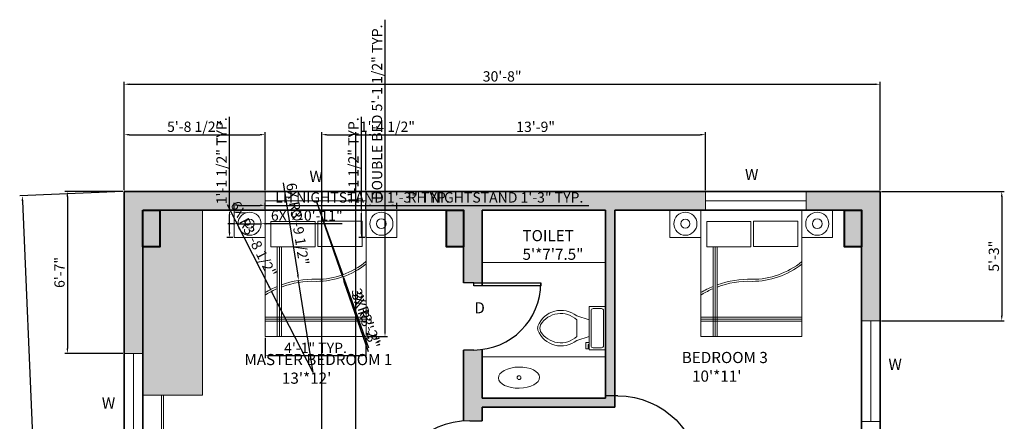
# Model space of a CAD drawing. Units: inches. Extents: x 351 to 1945, y 4338 to 4989.
# Tile 3 of 4: x 351 to 830, y 4716 to 4912. Entities that reach past the tile are written whole.
import ezdxf

# ---------------------------------------------------------------- set-up
doc = ezdxf.new("R2010")
doc.units = ezdxf.units.IN
for name, color, linetype, lineweight in [('A-ANNO-DIMS', 55, 'Continuous', 18), ('A-ANNO-IDEN', 55, 'Continuous', 18), ('A-AREA-IDEN', 55, 'Continuous', 18), ('A-COLS-PATT', 210, 'Continuous', 13), ('A-FLOR-CASE', 30, 'Continuous', 20), ('A-FLOR-CASE-PATT', 30, 'Continuous', 13), ('A-FLOR-FIXT', 9, 'Continuous', 18), ('A-WALL-PATT', 130, 'Continuous', 13), ('COLUMN', 210, 'Continuous', 40), ('DOOR', 52, 'Continuous', 25), ('FUR', 142, 'Continuous', 18), ('WALL', 130, 'Continuous', 35), ('WIND', 10, 'Continuous', 20)]:
    doc.layers.add(name, color=color, linetype=linetype, lineweight=lineweight)
doc.styles.get("Standard").update_dxf_attribs({"font": 'arial.ttf'})
doc.dimstyles.new('ISO-25', dxfattribs={"dimtxt": 5, "dimasz": 2.5, "dimexe": 1.25, "dimexo": 0.625, "dimtad": 1, "dimdec": 0, "dimlunit": 4, "dimtxsty": 'Standard', "dimcen": 2.5, "dimadec": 0, "dimazin": 0, "dimtfac": 1, "dimtdec": 0, "dimtmove": 0, "dimatfit": 3, "dimfxl": 1, "dimarcsym": 0})

# ---------------------------------------------------------------- blocks, each defined once
blk = doc.blocks.new('*U2')
for p, q in [((0, 0), (0, -6)), ((40, 0), (40, -6))]:
    blk.add_line(p, q)
blk.add_lwpolyline([(0, 0), (0, 40), (1.75, 40), (1.75, 0)], close=True)
blk.add_arc((0, 0), 40, 0, 90)
blk = doc.blocks.new('*U4')
for p, q in [((9.5, -6), (9.5, -2)), ((-10, -8.5), (-8, -8.5)), ((-10, -9.5), (-10, -8.5)), ((-7, -9.5), (-10, -9.5)), ((-8, -8.5), (-8, -8)), ((-7, -8), (-7, -9.5)), ((-4, -8), (-6, -14)), ((4, -8), (6, -14)), ((4, -14), (-4, -14))]:
    blk.add_line(p, q)
blk.add_lwpolyline([(10.5, -8), (10.5, 0), (-10.5, 0), (-10.5, -8)], close=True)
for points in [[(-9.5, -2), (-9.5, -6)], [(8.5, -1), (-8.5, -1)], [(-8.5, -7), (8.5, -7)]]:
    blk.add_lwpolyline(points)
for centre, radius, start, end in [((-8.62, -1.88), 0.884, 81.8699, 188.1301), ((8.62, -1.88), 0.884, 351.8699, 98.1301), ((-8.62, -6.12), 0.884, 171.8699, 278.1301), ((8.62, -6.12), 0.884, 261.8699, 8.1301), ((3.52, -21.58), 12.17, 141.4691, 247.9714), ((4.2, -21.82), 11.33, 136.3677, 238.9468), ((-3.52, -21.58), 12.17, 292.0284, 38.5307), ((-4.2, -21.82), 11.33, 301.053, 43.6321), ((0, -27.88), 4, 245.7318, 294.2682), ((0, -29), 4, 254.8605, 285.1395)]:
    blk.add_arc(centre, radius, start, end)
blk = doc.blocks.new('*D5')
at = {"layer": 'A-ANNO-DIMS', "color": 0, "lineweight": -2, "transparency": 16777216}
for p, q in [((402.08, 4828.78), (402.08, 4881.59)), ((404.58, 4880.34), (767.08, 4880.34)), ((769.58, 4828.78), (769.58, 4881.59))]:
    blk.add_line(p, q, dxfattribs=at)
at = {"layer": 'A-ANNO-DIMS', "color": 0, "lineweight": 100, "transparency": 16777216}
for points in [[(404.58, 4880.75), (404.58, 4879.92), (402.08, 4880.34)], [(767.08, 4880.75), (767.08, 4879.92), (769.58, 4880.34)]]:
    blk.add_solid(points, dxfattribs=at)
at = {"layer": 'Defpoints', "color": 0, "lineweight": 100, "transparency": 16777216}
for p in [(769.58, 4880.34), (402.08, 4828.16), (769.58, 4828.16)]:
    blk.add_point(p, dxfattribs=at)
at = {"layer": 'A-ANNO-DIMS', "color": 0, "transparency": 16777216, "insert": (585.83, 4883.52), "char_height": 5, "attachment_point": 5}
blk.add_mtext('30\'-8"', dxfattribs=at)
blk = doc.blocks.new('*D6')
at = {"layer": 'A-ANNO-DIMS', "color": 0, "lineweight": -2, "transparency": 16777216}
for p, q in [((401.46, 4828.13), (351.25, 4825.99)), ((352.6, 4823.54), (371.89, 4372.54)), ((420.96, 4372.13), (370.75, 4369.99))]:
    blk.add_line(p, q, dxfattribs=at)
at = {"layer": 'A-ANNO-DIMS', "color": 0, "lineweight": 100, "transparency": 16777216}
for points in [[(353.02, 4823.56), (352.19, 4823.52), (352.5, 4826.04)], [(372.31, 4372.55), (371.48, 4372.52), (372, 4370.04)]]:
    blk.add_solid(points, dxfattribs=at)
at = {"layer": 'Defpoints', "color": 0, "lineweight": 100, "transparency": 16777216}
for p in [(402.08, 4828.16), (421.58, 4372.16), (372, 4370.04)]:
    blk.add_point(p, dxfattribs=at)
at = {"layer": 'A-ANNO-DIMS', "color": 0, "transparency": 16777216, "insert": (365.42, 4598.17), "char_height": 5, "attachment_point": 5, "rotation": 272.4487}
blk.add_mtext("38'", dxfattribs=at)
blk = doc.blocks.new('BED-DOUBLE')
for p, q in [((5.95, 43.76), (5.95, 0)), ((6.95, 43.76), (6.95, 0)), ((7.95, 43.76), (7.95, 0)), ((0.52, 20.56), (0, 20.22)), ((0, 9.54), (49.08, 9.54)), ((0, 8.54), (49.08, 8.54)), ((0, 7.54), (49.08, 7.54))]:
    blk.add_line(p, q)
for points in [[(0, 61.61), (49.08, 61.61), (49.08, 0), (0, 0)], [(2.84, 55.99), (24.35, 55.99), (24.35, 43.76), (2.84, 43.76)], [(25.67, 56.16), (47.18, 56.16), (47.18, 43.92), (25.67, 43.92)]]:
    blk.add_lwpolyline(points, close=True)
for centre, radius, start, end in [((24.92, 66.13), 38.24, 270, 309.1724), ((24.92, 66.13), 39.24, 270, 307.9925), ((23.4, -17.42), 45.34, 112.6404, 121.0693), ((23.4, -17.42), 45.34, 88.0757, 109.9277), ((23.4, -17.42), 44.34, 88.0757, 110.3969), ((23.4, -17.42), 44.34, 113.1804, 121.0693)]:
    blk.add_arc(centre, radius, start, end)
blk = doc.blocks.new('NIGHTSTAND-R')
blk.add_lwpolyline([(0, 13.33), (15.02, 13.33), (15.02, 0), (0, 0)], close=True)
for radius in [5.61, 2.37]:
    blk.add_circle((7.51, 6.66), radius)
blk = doc.blocks.new('NIGHTSTAND-L')
blk.add_lwpolyline([(0, 13.33), (15.02, 13.33), (15.02, 0), (0, 0)], close=True)
for radius in [5.61, 2.18]:
    blk.add_circle((7.51, 6.66), radius)
blk = doc.blocks.new('WIN-49')
blk.add_line((0, 4.5), (49.03, 4.5))
blk.add_lwpolyline([(0, 0), (49.03, 0), (49.03, 9), (0, 9)], close=True)
blk = doc.blocks.new('*D21')
at = {"layer": 'A-ANNO-DIMS', "color": 0, "lineweight": -2, "transparency": 16777216}
for p, q in [((528.87, 4819.16), (528.87, 4911.76)), ((520.25, 4819.16), (530.12, 4819.16)), ((528.87, 4760.05), (528.87, 4816.66)), ((520.25, 4757.55), (530.12, 4757.55))]:
    blk.add_line(p, q, dxfattribs=at)
at = {"layer": 'A-ANNO-DIMS', "color": 0, "lineweight": 100, "transparency": 16777216}
for points in [[(528.45, 4816.66), (529.28, 4816.66), (528.87, 4819.16)], [(528.45, 4760.05), (529.28, 4760.05), (528.87, 4757.55)]]:
    blk.add_solid(points, dxfattribs=at)
at = {"layer": 'Defpoints', "color": 0, "lineweight": 100, "transparency": 16777216}
for p in [(519.62, 4819.16), (528.87, 4819.16), (519.62, 4757.55)]:
    blk.add_point(p, dxfattribs=at)
at = {"layer": 'A-ANNO-DIMS', "color": 0, "transparency": 16777216, "insert": (525.65, 4866.71), "char_height": 5, "attachment_point": 5, "rotation": 90}
blk.add_mtext('DOUBLE BED 5\'-1 1/2" TYP.', dxfattribs=at)
blk = doc.blocks.new('*D22')
at = {"layer": 'A-ANNO-DIMS', "color": 0, "lineweight": -2, "transparency": 16777216}
for p, q in [((470.55, 4756.92), (470.55, 4747.06)), ((519.62, 4756.92), (519.62, 4747.06)), ((473.05, 4748.31), (517.12, 4748.31))]:
    blk.add_line(p, q, dxfattribs=at)
at = {"layer": 'A-ANNO-DIMS', "color": 0, "lineweight": 100, "transparency": 16777216}
for points in [[(473.05, 4748.72), (473.05, 4747.89), (470.55, 4748.31)], [(517.12, 4748.72), (517.12, 4747.89), (519.62, 4748.31)]]:
    blk.add_solid(points, dxfattribs=at)
at = {"layer": 'Defpoints', "color": 0, "lineweight": 100, "transparency": 16777216}
for p in [(470.55, 4757.55), (519.62, 4757.55), (519.62, 4748.31)]:
    blk.add_point(p, dxfattribs=at)
at = {"layer": 'A-ANNO-DIMS', "color": 0, "transparency": 16777216, "insert": (495.09, 4751.44), "char_height": 5, "attachment_point": 5}
blk.add_mtext('4\'-1" TYP.', dxfattribs=at)
blk = doc.blocks.new('*D23')
at = {"layer": 'A-ANNO-DIMS', "color": 0, "lineweight": -2, "transparency": 16777216}
for p, q in [((519.62, 4819.78), (519.62, 4822.66)), ((522.12, 4821.41), (532.15, 4821.41)), ((534.65, 4819.78), (534.65, 4822.66)), ((534.65, 4821.41), (627.99, 4821.41))]:
    blk.add_line(p, q, dxfattribs=at)
at = {"layer": 'A-ANNO-DIMS', "color": 0, "lineweight": 100, "transparency": 16777216}
for points in [[(522.12, 4821.83), (522.12, 4821), (519.62, 4821.41)], [(532.15, 4821.83), (532.15, 4821), (534.65, 4821.41)]]:
    blk.add_solid(points, dxfattribs=at)
at = {"layer": 'Defpoints', "color": 0, "lineweight": 100, "transparency": 16777216}
for p in [(534.65, 4821.41), (519.62, 4819.16), (534.65, 4819.16)]:
    blk.add_point(p, dxfattribs=at)
at = {"layer": 'A-ANNO-DIMS', "color": 0, "transparency": 16777216, "insert": (582.57, 4824.62), "char_height": 5, "attachment_point": 5}
blk.add_mtext('RH NIGHTSTAND 1\'-3" TYP.', dxfattribs=at)
blk = doc.blocks.new('*D24')
at = {"layer": 'A-ANNO-DIMS', "color": 0, "lineweight": -2, "transparency": 16777216}
for p, q in [((517.37, 4819.16), (517.37, 4864.57)), ((519, 4819.16), (516.12, 4819.16)), ((517.37, 4808.33), (517.37, 4816.66)), ((519, 4805.83), (516.12, 4805.83))]:
    blk.add_line(p, q, dxfattribs=at)
at = {"layer": 'A-ANNO-DIMS', "color": 0, "lineweight": 100, "transparency": 16777216}
for points in [[(516.95, 4816.66), (517.79, 4816.66), (517.37, 4819.16)], [(516.95, 4808.33), (517.79, 4808.33), (517.37, 4805.83)]]:
    blk.add_solid(points, dxfattribs=at)
at = {"layer": 'Defpoints', "color": 0, "lineweight": 100, "transparency": 16777216}
for p in [(517.37, 4819.16), (519.62, 4819.16), (519.62, 4805.83)]:
    blk.add_point(p, dxfattribs=at)
at = {"layer": 'A-ANNO-DIMS', "color": 0, "transparency": 16777216, "insert": (514.16, 4843.11), "char_height": 5, "attachment_point": 5, "rotation": 90}
blk.add_mtext('1\'-1 1/2" TYP.', dxfattribs=at)
blk = doc.blocks.new('*D25')
at = {"layer": 'A-ANNO-DIMS', "color": 0, "lineweight": -2, "transparency": 16777216}
for p, q in [((455.53, 4819.78), (455.53, 4822.66)), ((458.03, 4821.41), (468.05, 4821.41)), ((470.55, 4819.78), (470.55, 4822.66)), ((470.55, 4821.41), (562.77, 4821.41))]:
    blk.add_line(p, q, dxfattribs=at)
at = {"layer": 'A-ANNO-DIMS', "color": 0, "lineweight": 100, "transparency": 16777216}
for points in [[(458.03, 4821.83), (458.03, 4821), (455.53, 4821.41)], [(468.05, 4821.83), (468.05, 4821), (470.55, 4821.41)]]:
    blk.add_solid(points, dxfattribs=at)
at = {"layer": 'Defpoints', "color": 0, "lineweight": 100, "transparency": 16777216}
for p in [(470.55, 4821.41), (455.53, 4819.16), (470.55, 4819.16)]:
    blk.add_point(p, dxfattribs=at)
at = {"layer": 'A-ANNO-DIMS', "color": 0, "transparency": 16777216, "insert": (517.91, 4824.62), "char_height": 5, "attachment_point": 5}
blk.add_mtext('LH NIGHTSTAND 1\'-3" TYP.', dxfattribs=at)
blk = doc.blocks.new('*D26')
at = {"layer": 'A-ANNO-DIMS', "color": 0, "lineweight": -2, "transparency": 16777216}
for p, q in [((453.27, 4819.16), (453.27, 4864.57)), ((454.9, 4819.16), (452.02, 4819.16)), ((453.27, 4808.33), (453.27, 4816.66)), ((454.9, 4805.83), (452.02, 4805.83))]:
    blk.add_line(p, q, dxfattribs=at)
at = {"layer": 'A-ANNO-DIMS', "color": 0, "lineweight": 100, "transparency": 16777216}
for points in [[(452.86, 4816.66), (453.69, 4816.66), (453.27, 4819.16)], [(452.86, 4808.33), (453.69, 4808.33), (453.27, 4805.83)]]:
    blk.add_solid(points, dxfattribs=at)
at = {"layer": 'Defpoints', "color": 0, "lineweight": 100, "transparency": 16777216}
for p in [(453.27, 4819.16), (455.53, 4819.16), (455.53, 4805.83)]:
    blk.add_point(p, dxfattribs=at)
at = {"layer": 'A-ANNO-DIMS', "color": 0, "transparency": 16777216, "insert": (450.06, 4843.11), "char_height": 5, "attachment_point": 5, "rotation": 90}
blk.add_mtext('1\'-1 1/2" TYP.', dxfattribs=at)
blk = doc.blocks.new('*D33')
at = {"layer": 'A-ANNO-DIMS', "color": 0, "lineweight": -2, "transparency": 16777216}
for p, q in [((402.08, 4828.78), (402.08, 4857.06)), ((404.58, 4855.81), (468.05, 4855.81)), ((470.55, 4828.78), (470.55, 4857.06))]:
    blk.add_line(p, q, dxfattribs=at)
at = {"layer": 'A-ANNO-DIMS', "color": 0, "lineweight": 100, "transparency": 16777216}
for points in [[(404.58, 4856.23), (404.58, 4855.39), (402.08, 4855.81)], [(468.05, 4856.23), (468.05, 4855.39), (470.55, 4855.81)]]:
    blk.add_solid(points, dxfattribs=at)
at = {"layer": 'Defpoints', "color": 0, "lineweight": 100, "transparency": 16777216}
for p in [(470.55, 4855.81), (402.08, 4828.16), (470.55, 4828.16)]:
    blk.add_point(p, dxfattribs=at)
at = {"layer": 'A-ANNO-DIMS', "color": 0, "transparency": 16777216, "insert": (436.32, 4859.02), "char_height": 5, "attachment_point": 5}
blk.add_mtext('5\'-8 1/2"', dxfattribs=at)
blk = doc.blocks.new('*D34')
at = {"layer": 'A-ANNO-DIMS', "color": 0, "lineweight": -2, "transparency": 16777216}
for p, q in [((519.58, 4828.78), (519.58, 4857.06)), ((522.08, 4855.81), (682.13, 4855.81)), ((684.63, 4828.78), (684.63, 4857.06))]:
    blk.add_line(p, q, dxfattribs=at)
at = {"layer": 'A-ANNO-DIMS', "color": 0, "lineweight": 100, "transparency": 16777216}
for points in [[(522.08, 4856.23), (522.08, 4855.39), (519.58, 4855.81)], [(682.13, 4856.23), (682.13, 4855.39), (684.63, 4855.81)]]:
    blk.add_solid(points, dxfattribs=at)
at = {"layer": 'Defpoints', "color": 0, "lineweight": 100, "transparency": 16777216}
for p in [(684.63, 4855.81), (519.58, 4828.16), (684.63, 4828.16)]:
    blk.add_point(p, dxfattribs=at)
at = {"layer": 'A-ANNO-DIMS', "color": 0, "transparency": 16777216, "insert": (602.1, 4858.99), "char_height": 5, "attachment_point": 5}
blk.add_mtext('13\'-9"', dxfattribs=at)
blk = doc.blocks.new('*D35')
at = {"layer": 'A-ANNO-DIMS', "color": 0, "lineweight": -2, "transparency": 16777216}
for p, q in [((401.46, 4828.16), (373.18, 4828.16)), ((374.43, 4825.66), (374.43, 4751.91)), ((401.46, 4749.41), (373.18, 4749.41))]:
    blk.add_line(p, q, dxfattribs=at)
at = {"layer": 'A-ANNO-DIMS', "color": 0, "lineweight": 100, "transparency": 16777216}
for points in [[(374.02, 4825.66), (374.85, 4825.66), (374.43, 4828.16)], [(374.02, 4751.91), (374.85, 4751.91), (374.43, 4749.41)]]:
    blk.add_solid(points, dxfattribs=at)
at = {"layer": 'Defpoints', "color": 0, "lineweight": 100, "transparency": 16777216}
for p in [(402.08, 4828.16), (374.43, 4749.41), (402.08, 4749.41)]:
    blk.add_point(p, dxfattribs=at)
at = {"layer": 'A-ANNO-DIMS', "color": 0, "transparency": 16777216, "insert": (371.26, 4788.78), "char_height": 5, "attachment_point": 5, "rotation": 90}
blk.add_mtext('6\'-7"', dxfattribs=at)
blk = doc.blocks.new('*D37')
at = {"layer": 'A-ANNO-DIMS', "color": 0, "lineweight": -2, "transparency": 16777216}
for p, q in [((770.21, 4828.16), (829.98, 4828.16)), ((828.73, 4825.66), (828.73, 4767.73)), ((770.21, 4765.23), (829.98, 4765.23))]:
    blk.add_line(p, q, dxfattribs=at)
at = {"layer": 'A-ANNO-DIMS', "color": 0, "lineweight": 100, "transparency": 16777216}
for points in [[(828.32, 4825.66), (829.15, 4825.66), (828.73, 4828.16)], [(828.32, 4767.73), (829.15, 4767.73), (828.73, 4765.23)]]:
    blk.add_solid(points, dxfattribs=at)
at = {"layer": 'Defpoints', "color": 0, "lineweight": 100, "transparency": 16777216}
for p in [(769.58, 4828.16), (769.58, 4765.23), (828.73, 4765.23)]:
    blk.add_point(p, dxfattribs=at)
at = {"layer": 'A-ANNO-DIMS', "color": 0, "transparency": 16777216, "insert": (825.56, 4796.69), "char_height": 5, "attachment_point": 5, "rotation": 90}
blk.add_mtext('5\'-3"', dxfattribs=at)
blk = doc.blocks.new('*D39')
at = {"layer": 'A-ANNO-DIMS', "color": 0, "lineweight": -2, "transparency": 16777216}
for p, q in [((498.08, 4372.78), (498.08, 4857.06)), ((500.58, 4855.81), (512.17, 4855.81)), ((514.67, 4372.78), (514.67, 4857.06)), ((514.67, 4855.81), (542.89, 4855.81))]:
    blk.add_line(p, q, dxfattribs=at)
at = {"layer": 'A-ANNO-DIMS', "color": 0, "lineweight": 100, "transparency": 16777216}
for points in [[(500.58, 4856.23), (500.58, 4855.39), (498.08, 4855.81)], [(512.17, 4856.23), (512.17, 4855.39), (514.67, 4855.81)]]:
    blk.add_solid(points, dxfattribs=at)
at = {"layer": 'Defpoints', "color": 0, "lineweight": 100, "transparency": 16777216}
for p in [(514.67, 4855.81), (498.08, 4372.16), (514.67, 4372.16)]:
    blk.add_point(p, dxfattribs=at)
at = {"layer": 'A-ANNO-DIMS', "color": 0, "transparency": 16777216, "insert": (530.03, 4859.02), "char_height": 5, "attachment_point": 5}
blk.add_mtext('1\'-4 1/2"', dxfattribs=at)
blk = doc.blocks.new('*D53')
at = {"layer": 'A-ANNO-DIMS', "color": 0, "lineweight": -2, "transparency": 16777216}
for p, q in [((454.92, 4812.5), (452.42, 4812.5)), ((457.42, 4812.49), (468.65, 4812.49)), ((508.02, 4812.49), (471.15, 4812.49))]:
    blk.add_line(p, q, dxfattribs=at)
at = {"layer": 'A-ANNO-DIMS', "color": 0, "lineweight": 100, "transparency": 16777216}
for points in [[(454.92, 4812.91), (454.92, 4812.08), (457.42, 4812.49)], [(471.15, 4812.91), (471.15, 4812.08), (468.65, 4812.49)]]:
    blk.add_solid(points, dxfattribs=at)
at = {"layer": 'Defpoints', "color": 0, "lineweight": 100, "transparency": 16777216}
for p in [(457.42, 4812.49), (468.65, 4812.49)]:
    blk.add_point(p, dxfattribs=at)
at = {"layer": 'A-ANNO-DIMS', "color": 0, "transparency": 16777216, "insert": (490.84, 4815.81), "char_height": 5, "attachment_point": 5, "rotation": 359.9951}
blk.add_mtext('6X ∅0\'-11"', dxfattribs=at)
blk = doc.blocks.new('*D54')
at = {"layer": 'A-ANNO-DIMS', "color": 0, "lineweight": -2, "transparency": 16777216}
for p, q in [((479.33, 4832.39), (486.46, 4787.38)), ((493.95, 4740.12), (486.85, 4784.91))]:
    blk.add_line(p, q, dxfattribs=at)
at = {"layer": 'A-ANNO-DIMS', "color": 0, "lineweight": 100, "transparency": 16777216}
blk.add_solid([(486.87, 4787.44), (486.05, 4787.31), (486.85, 4784.91)], dxfattribs=at)
at = {"layer": 'Defpoints', "color": 0, "lineweight": 100, "transparency": 16777216}
for p in [(486.85, 4784.91), (493.95, 4740.12)]:
    blk.add_point(p, dxfattribs=at)
at = {"layer": 'A-ANNO-DIMS', "color": 0, "transparency": 16777216, "insert": (485.77, 4812.28), "char_height": 5, "attachment_point": 5, "rotation": 279.0021}
blk.add_mtext('6X R3\'-9 1/2"', dxfattribs=at)
blk = doc.blocks.new('*D55')
at = {"layer": 'A-ANNO-DIMS', "color": 0, "lineweight": -2, "transparency": 16777216}
for p, q in [((452.08, 4821.84), (472.59, 4781.81)), ((493.95, 4740.12), (473.73, 4779.59))]:
    blk.add_line(p, q, dxfattribs=at)
at = {"layer": 'A-ANNO-DIMS', "color": 0, "lineweight": 100, "transparency": 16777216}
blk.add_solid([(472.96, 4782), (472.22, 4781.62), (473.73, 4779.59)], dxfattribs=at)
at = {"layer": 'Defpoints', "color": 0, "lineweight": 100, "transparency": 16777216}
for p in [(473.73, 4779.59), (493.95, 4740.12)]:
    blk.add_point(p, dxfattribs=at)
at = {"layer": 'A-ANNO-DIMS', "color": 0, "transparency": 16777216, "insert": (464.46, 4804.73), "char_height": 5, "attachment_point": 5, "rotation": 297.1254}
blk.add_mtext('6X R3\'-8 1/2"', dxfattribs=at)
blk = doc.blocks.new('*D56')
at = {"layer": 'A-ANNO-DIMS', "color": 0, "lineweight": -2, "transparency": 16777216}
for p, q in [((495.47, 4823.68), (508.24, 4786.58)), ((520.8, 4750.1), (509.06, 4784.21))]:
    blk.add_line(p, q, dxfattribs=at)
at = {"layer": 'A-ANNO-DIMS', "color": 0, "lineweight": 100, "transparency": 16777216}
blk.add_solid([(509.45, 4784.35), (508.66, 4784.08), (508.24, 4786.58)], dxfattribs=at)
at = {"layer": 'Defpoints', "color": 0, "lineweight": 100, "transparency": 16777216}
for p in [(495.47, 4823.68), (508.24, 4786.58)]:
    blk.add_point(p, dxfattribs=at)
at = {"layer": 'A-ANNO-DIMS', "color": 0, "transparency": 16777216, "insert": (518.91, 4765.35), "char_height": 5, "attachment_point": 5, "rotation": 288.9957}
blk.add_mtext('3X R3\'-3"', dxfattribs=at)
blk = doc.blocks.new('*D57')
at = {"layer": 'A-ANNO-DIMS', "color": 0, "lineweight": -2, "transparency": 16777216}
for p, q in [((495.47, 4823.68), (508.29, 4787.65)), ((521.02, 4751.87), (509.13, 4785.3))]:
    blk.add_line(p, q, dxfattribs=at)
at = {"layer": 'A-ANNO-DIMS', "color": 0, "lineweight": 100, "transparency": 16777216}
blk.add_solid([(509.52, 4785.44), (508.73, 4785.16), (508.29, 4787.65)], dxfattribs=at)
at = {"layer": 'Defpoints', "color": 0, "lineweight": 100, "transparency": 16777216}
for p in [(495.47, 4823.68), (508.29, 4787.65)]:
    blk.add_point(p, dxfattribs=at)
at = {"layer": 'A-ANNO-DIMS', "color": 0, "transparency": 16777216, "insert": (518.97, 4767.1), "char_height": 5, "attachment_point": 5, "rotation": 289.5856}
blk.add_mtext('3X R3\'-2"', dxfattribs=at)

msp = doc.modelspace()

# ---------------------------------------------------------------- hatches: boundary and pattern name
at = {"layer": 'A-COLS-PATT'}
h = msp.add_hatch(color=256, dxfattribs=at)
h.dxf.hatch_style = 1
h.paths.add_polyline_path([(419.45, 4819.16), (411.08, 4819.16), (411.08, 4801.31), (419.45, 4801.31)])
h.paths.add_polyline_path([(760.58, 4819.16), (752.22, 4819.16), (752.22, 4801.31), (760.58, 4801.31)])
h.paths.add_polyline_path([(567.08, 4819.16), (558.72, 4819.16), (558.72, 4801.31), (567.08, 4801.31)])
h.paths.add_polyline_path([(423.85, 4675.88), (411.08, 4675.88), (411.08, 4669.65), (423.85, 4669.65)])
h.paths.add_polyline_path([(575.47, 4670.66), (567.1, 4670.66), (567.1, 4658.77), (575.47, 4658.77)])
h.paths.add_polyline_path([(575.47, 4676.62), (570.08, 4676.62), (567.1, 4676.62), (567.1, 4670.66), (575.47, 4670.66)])
h.paths.add_polyline_path([(769.58, 4687.16), (751.73, 4687.16), (751.73, 4682.66), (769.58, 4682.66)])
h.paths.add_polyline_path([(769.58, 4682.66), (751.73, 4682.66), (751.73, 4678.79), (769.58, 4678.79)])
h.paths.add_polyline_path([(514.67, 4381.16), (502.58, 4381.16), (502.58, 4372.16), (514.67, 4372.16)])
h.paths.add_polyline_path([(624.15, 4381.16), (606.3, 4381.16), (606.3, 4372.16), (624.15, 4372.16)])
h.paths.add_polyline_path([(752.08, 4381.16), (734.23, 4381.16), (734.23, 4372.16), (752.08, 4372.16)])
h.paths.add_polyline_path([(684.94, 4526.8), (676.58, 4526.8), (676.58, 4508.95), (684.94, 4508.95)])
h.paths.add_polyline_path([(419.45, 4492.01), (411.08, 4492.01), (411.08, 4474.16), (419.45, 4474.16)])
h.paths.add_polyline_path([(414.54, 4480.61), (443.82, 4480.61), (443.82, 4500.88), (414.54, 4500.88)], flags=9)
at = {"layer": 'A-FLOR-CASE-PATT'}
h = msp.add_hatch(color=256, dxfattribs=at)
h.dxf.hatch_style = 1
h.paths.add_polyline_path([(440.18, 4819.16), (419.45, 4819.16), (419.45, 4801.31), (411.08, 4801.31), (411.08, 4729.12), (440.18, 4729.12)])
h.paths.add_polyline_path([(760.58, 4704.97), (709.51, 4704.97), (709.51, 4687.16), (760.58, 4687.16)])
h.paths.add_polyline_path([(555.08, 4624.13), (533.62, 4624.13), (533.62, 4538.66), (546.72, 4538.66), (546.72, 4556.51), (555.08, 4556.51)])
at = {"layer": 'A-WALL-PATT'}
h = msp.add_hatch(color=256, dxfattribs=at)
h.dxf.hatch_style = 1
h.paths.add_polyline_path([(519.58, 4828.16), (519.58, 4819.16), (534.65, 4819.16), (567.08, 4819.16), (567.08, 4801.31), (567.08, 4783.74), (571.99, 4783.74), (576.08, 4783.74), (576.08, 4819.16), (636.08, 4819.16), (636.08, 4728.72), (640.58, 4728.72), (640.58, 4819.16), (684.63, 4819.16), (684.63, 4828.16), (640.58, 4828.16), (576.08, 4828.16)])
h.paths.add_polyline_path([(402.08, 4828.16), (402.08, 4749.41), (411.08, 4749.41), (411.08, 4819.16), (419.45, 4819.16), (470.55, 4819.16), (470.55, 4828.16)])
h.paths.add_polyline_path([(733.65, 4828.16), (733.65, 4819.16), (746.53, 4819.16), (760.58, 4819.16), (760.58, 4801.31), (760.58, 4765.23), (769.58, 4765.23), (769.58, 4828.16)])
h.paths.add_polyline_path([(402.08, 4670.66), (402.08, 4623.83), (411.08, 4623.83), (411.08, 4670.66), (411.08, 4675.88), (411.08, 4700.38), (402.08, 4700.38)])
h.paths.add_polyline_path([(555.08, 4670.66), (555.08, 4667.68), (559.58, 4667.68), (559.58, 4670.66), (567.1, 4670.66), (567.1, 4675.16), (423.95, 4675.16), (423.85, 4675.16), (423.85, 4670.66)])
h.paths.add_polyline_path([(576.08, 4727.66), (576.08, 4751.3, -0.031413), (571.99, 4751.04), (567.08, 4751.04), (567.08, 4716.51, -0.01877), (570.08, 4716.62), (576.08, 4716.62), (576.08, 4723.16), (636.08, 4723.16), (640.58, 4723.16), (640.58, 4728.72), (636.08, 4728.72), (636.08, 4727.66)])
h.paths.add_polyline_path([(672.08, 4682.66), (672.08, 4641.87), (676.58, 4641.87), (676.58, 4682.66), (724.58, 4682.66), (724.58, 4677.41), (729.08, 4677.41), (729.08, 4682.66), (751.73, 4682.66), (751.73, 4687.16), (709.51, 4687.16), (684.61, 4687.16), (640.58, 4687.16), (640.58, 4688.72), (636.08, 4688.72), (636.08, 4682.66)])
h.paths.add_polyline_path([(753.8, 4463.91), (782.66, 4463.91), (782.66, 4484.16), (753.8, 4484.16)], flags=9)
h.paths.add_polyline_path([(760.86, 4391.5), (776.24, 4391.5), (776.24, 4411.77), (760.86, 4411.77)], flags=9)
h.paths.add_polyline_path([(690.04, 4455.43), (720.56, 4455.43), (720.56, 4475.7), (690.04, 4475.7)], flags=9)
h.paths.add_polyline_path([(676.19, 4400.06), (720.94, 4400.06), (720.94, 4420.3), (676.19, 4420.3)], flags=9)
h.paths.add_polyline_path([(550.38, 4425.45), (615.73, 4425.45), (615.73, 4445.72), (550.38, 4445.72)], flags=9)
h.paths.add_polyline_path([(417.92, 4480.61), (447.2, 4480.61), (447.2, 4500.88), (417.92, 4500.88)], flags=9)
h.paths.add_polyline_path([(449.69, 4582.66), (497.94, 4582.66), (497.94, 4602.93), (449.69, 4602.93)], flags=9)
h.paths.add_polyline_path([(580.8, 4638.02), (622.18, 4638.02), (622.18, 4658.29), (580.8, 4658.29)], flags=9)
h.paths.add_polyline_path([(748.64, 4653.12), (792.13, 4653.12), (792.13, 4673.39), (748.64, 4673.39)], flags=9)
h.paths.add_polyline_path([(686.44, 4648.7), (715.72, 4648.7), (715.72, 4668.97), (686.44, 4668.97)], flags=25)
h.paths.add_polyline_path([(689.64, 4550.87), (725.93, 4550.87), (725.93, 4571.14), (689.64, 4571.14)], flags=9)
h.paths.add_polyline_path([(671.27, 4732.55), (719.52, 4732.55), (719.52, 4752.82), (671.27, 4752.82)], flags=9)
h.paths.add_polyline_path([(458.57, 4731.55), (540.55, 4731.55), (540.55, 4751.82), (458.57, 4751.82)], flags=9)
h = msp.add_hatch(color=256, dxfattribs=at)
h.dxf.hatch_style = 1
h.paths.add_polyline_path([(729.08, 4663.38), (724.58, 4663.38), (724.58, 4610.66), (676.58, 4610.66), (676.58, 4612.12), (676.55, 4612.12), (672.08, 4612.12), (672.08, 4606.16), (672.08, 4581.14), (676.58, 4581.14), (676.58, 4606.16), (729.08, 4606.16), (730.91, 4606.16), (730.91, 4610.66), (729.08, 4610.66)])
h.paths.add_polyline_path([(676.58, 4507.65), (676.58, 4508.95), (676.58, 4508.95), (676.58, 4526.98), (672.08, 4526.98), (672.08, 4489.16), (676.58, 4489.16), (687.08, 4489.16), (747.58, 4489.16), (747.58, 4445.66), (742.58, 4445.66), (687.08, 4445.66), (676.58, 4445.66), (672.08, 4445.66), (672.08, 4424.71), (676.58, 4424.71), (676.58, 4441.16), (687.08, 4441.16), (747.08, 4441.16), (747.08, 4423.66), (752.08, 4423.66), (752.08, 4445.66), (752.08, 4458.62), (752.08, 4489.16), (752.08, 4493.66), (676.58, 4493.66)])
h.paths.add_polyline_path([(734.23, 4381.16), (687.08, 4381.16), (680.85, 4381.16), (624.15, 4381.16), (624.15, 4372.16), (687.08, 4372.16), (734.23, 4372.16)])
h.paths.add_polyline_path([(606.3, 4381.16), (570.36, 4381.16), (563.7, 4381.16), (563.7, 4372.16), (606.3, 4372.16)])
h.paths.add_polyline_path([(753.8, 4463.91), (782.66, 4463.91), (782.66, 4484.16), (753.8, 4484.16)], flags=9)
h.paths.add_polyline_path([(760.86, 4391.5), (776.24, 4391.5), (776.24, 4411.77), (760.86, 4411.77)], flags=9)
h.paths.add_polyline_path([(690.04, 4455.43), (720.56, 4455.43), (720.56, 4475.7), (690.04, 4475.7)], flags=25)
h.paths.add_polyline_path([(676.19, 4400.06), (720.94, 4400.06), (720.94, 4420.3), (676.19, 4420.3)], flags=9)
h.paths.add_polyline_path([(550.38, 4425.45), (615.73, 4425.45), (615.73, 4445.72), (550.38, 4445.72)], flags=9)
h.paths.add_polyline_path([(417.92, 4480.61), (447.2, 4480.61), (447.2, 4500.88), (417.92, 4500.88)], flags=9)
h.paths.add_polyline_path([(449.69, 4582.66), (497.94, 4582.66), (497.94, 4602.93), (449.69, 4602.93)], flags=9)
h.paths.add_polyline_path([(580.8, 4638.02), (622.18, 4638.02), (622.18, 4658.29), (580.8, 4658.29)], flags=9)
h.paths.add_polyline_path([(748.64, 4653.12), (792.13, 4653.12), (792.13, 4673.39), (748.64, 4673.39)], flags=9)
h.paths.add_polyline_path([(686.44, 4648.7), (715.72, 4648.7), (715.72, 4668.97), (686.44, 4668.97)], flags=9)
h.paths.add_polyline_path([(689.64, 4550.87), (725.93, 4550.87), (725.93, 4571.14), (689.64, 4571.14)], flags=9)
h.paths.add_polyline_path([(671.27, 4732.55), (719.52, 4732.55), (719.52, 4752.82), (671.27, 4752.82)], flags=9)
h.paths.add_polyline_path([(594.05, 4791.87), (624.3, 4791.87), (624.3, 4812.11), (594.05, 4812.11)], flags=9)
h.paths.add_polyline_path([(458.57, 4731.55), (540.55, 4731.55), (540.55, 4751.82), (458.57, 4751.82)], flags=9)

# ---------------------------------------------------------------- linework, layer by layer
at = {"layer": 'A-FLOR-CASE'}
for p, q in [((440.18, 4819.16), (440.18, 4729.12)), ((440.18, 4729.12), (411.08, 4729.12)), ((420.12, 4729.12), (420.12, 4675.88)), ((421.12, 4729.12), (421.12, 4675.88))]:
    msp.add_line(p, q, dxfattribs=at)
at = {"layer": 'A-FLOR-FIXT'}
for p, q in [((576.08, 4793.55), (636.08, 4793.55)), ((576.08, 4747.79), (636.08, 4747.79))]:
    msp.add_line(p, q, dxfattribs=at)
msp.add_circle((594.04, 4737.62), 0.923, dxfattribs=at)
msp.add_ellipse((594.04, 4737.62), major_axis=(10.01, 0.2), ratio=0.514294, dxfattribs=at)
at = {"layer": 'COLUMN'}
for points in [[(411.08, 4819.16), (419.45, 4819.16), (419.45, 4801.31), (411.08, 4801.31)], [(558.72, 4819.16), (567.08, 4819.16), (567.08, 4801.31), (558.72, 4801.31)], [(752.22, 4819.16), (760.58, 4819.16), (760.58, 4801.31), (752.22, 4801.31)]]:
    msp.add_lwpolyline(points, close=True, dxfattribs=at)
at = {"layer": 'WALL'}
for p, q in [((402.08, 4828.16), (576.08, 4828.16)), ((402.08, 4670.66), (402.08, 4828.16)), ((576.08, 4828.16), (640.58, 4828.16)), ((640.58, 4828.16), (760.58, 4828.16)), ((640.58, 4828.16), (769.58, 4828.16)), ((769.58, 4828.16), (769.58, 4687.16)), ((411.08, 4819.16), (567.08, 4819.16)), ((411.08, 4675.16), (411.08, 4819.16)), ((567.08, 4819.16), (567.08, 4783.74)), ((576.08, 4819.16), (576.08, 4782.31)), ((576.08, 4819.16), (636.08, 4819.16)), ((636.08, 4819.16), (636.08, 4727.66)), ((640.58, 4819.16), (640.58, 4723.16)), ((640.58, 4819.16), (651.04, 4819.16)), ((640.58, 4819.16), (760.58, 4819.16)), ((760.58, 4819.16), (760.58, 4687.16)), ((567.08, 4751.04), (567.08, 4716.51)), ((576.08, 4751.3), (576.08, 4727.66)), ((636.08, 4727.66), (576.08, 4727.66)), ((636.08, 4723.16), (576.08, 4723.16)), ((576.08, 4723.16), (576.08, 4716.62)), ((636.08, 4723.16), (640.58, 4723.16))]:
    msp.add_line(p, q, dxfattribs=at)

# ---------------------------------------------------------------- block references
at = {"layer": 'A-FLOR-FIXT', "xscale": -1, "rotation": 270}
msp.add_blockref('*U4', (636.08, 4761.68), dxfattribs=at)
at = {"layer": 'DOOR', "xscale": 0.8173472156231275, "yscale": 0.8173472156231275, "zscale": 0.8173472156231275, "rotation": 270}
msp.add_blockref('*U2', (571.99, 4783.74), dxfattribs=at)
at = {"layer": 'DOOR', "xscale": -1, "rotation": 270}
msp.add_blockref('*U2', (642.08, 4688.72), dxfattribs=at)
at = {"layer": 'DOOR', "rotation": 90}
msp.add_blockref('*U2', (570.08, 4676.62), dxfattribs=at)
at = {"layer": 'FUR'}
for name, p in [('NIGHTSTAND-L', (455.53, 4805.83)), ('BED-DOUBLE', (470.55, 4757.55)), ('NIGHTSTAND-R', (519.62, 4805.83)), ('NIGHTSTAND-L', (667.41, 4805.83)), ('BED-DOUBLE', (682.43, 4757.55)), ('NIGHTSTAND-R', (731.51, 4805.83))]:
    msp.add_blockref(name, p, dxfattribs=at)
at = {"layer": 'WIND'}
for p in [(470.55, 4819.16), (684.63, 4819.16)]:
    msp.add_blockref('WIN-49', p, dxfattribs=at)
for p, rotation in [((760.58, 4765.23), 270.0000000000007), ((402.08, 4749.41), 270.0000000000006)]:
    msp.add_blockref('WIN-49', p, dxfattribs=dict(at, rotation=rotation))

# ---------------------------------------------------------------- texts
at = {"layer": 'A-ANNO-IDEN', "char_height": 5.43, "attachment_point": 1}
for s, insert in [('W', (492.13, 4838.22)), ('W', (703.91, 4839.17)), ('D', (572.32, 4774.3)), ('W', (773.64, 4746.79)), ('W', (391.19, 4727.95))]:
    msp.add_mtext_dynamic_manual_height_columns(s, width=132.0225, gutter_width=27.16, heights=[0], dxfattribs=dict(at, insert=insert))
at = {"layer": 'A-AREA-IDEN', "attachment_point": 1}
for s, insert, char_height in [('TOILET\\P5\'*7\'7.5"', (595.72, 4809.41), 5.432), ("MASTER BEDROOM 1\\P           13'*12'", (460.49, 4749.12), 5.4321), ("BEDROOM 3\\P   10'*11'", (673.18, 4750.12), 5.432)]:
    msp.add_mtext_dynamic_manual_height_columns(s, width=132.0225, gutter_width=27.16, heights=[0], dxfattribs=dict(at, insert=insert, char_height=char_height))

# ---------------------------------------------------------------- dimensions: what is measured, and where the dimension line sits
at = {"layer": 'A-ANNO-DIMS'}
for base, p1, p2, text, picture, middle in [((528.87, 4819.16), (519.62, 4757.55), (519.62, 4819.16), 'DOUBLE BED <> TYP.', '*D21', (525.65, 4866.71)), ((453.27, 4819.16), (455.53, 4805.83), (455.53, 4819.16), '<> TYP.', '*D26', (450.06, 4843.11)), ((517.37, 4819.16), (519.62, 4805.83), (519.62, 4819.16), '<> TYP.', '*D24', (514.16, 4843.11))]:
    dim = msp.add_linear_dim(base=base, p1=p1, p2=p2, angle=90, text=text, dimstyle='ISO-25', override={"dimdec": 1, "dimlfac": 1, "dimrnd": 0, "dimzin": 1, "dimdsep": 46, "dimlunit": 4, "dimfrac": 2}, dxfattribs=at)
    dim.commit()
    dim.dimension.update_dxf_attribs({"geometry": picture, "text_midpoint": middle})
for base, p1, p2, override, picture, middle in [((769.58484481, 4880.33818323), (402.08484481, 4828.15916803), (769.58484481, 4828.15916803), {"dimclrd": 0, "dimclre": 0, "dimclrt": 0}, '*D5', (585.83484481, 4883.51775349)), ((470.55, 4855.81), (402.08, 4828.16), (470.55, 4828.16), {"dimdec": 1, "dimlfac": 1, "dimrnd": 0, "dimzin": 1, "dimdsep": 46, "dimlunit": 4, "dimfrac": 2}, '*D33', (436.32, 4859.02)), ((514.67, 4855.81), (498.08, 4372.16), (514.67, 4372.16), {"dimdec": 1, "dimlfac": 1, "dimrnd": 0, "dimzin": 1, "dimdsep": 46, "dimlunit": 4, "dimfrac": 2}, '*D39', (530.03, 4859.02)), ((684.6266, 4855.8092), (519.5767, 4828.1592), (684.6266, 4828.1592), {"dimdec": 1, "dimlfac": 1, "dimrnd": 0, "dimzin": 1, "dimdsep": 46, "dimlunit": 4, "dimfrac": 2}, '*D34', (602.1016, 4858.9887))]:
    dim = msp.add_linear_dim(base=base, p1=p1, p2=p2, dimstyle='ISO-25', override=override, dxfattribs=at)
    dim.commit()
    dim.dimension.update_dxf_attribs({"geometry": picture, "text_midpoint": middle})
for base, p1, p2, text, picture, middle in [((470.55, 4821.41), (455.53, 4819.16), (470.55, 4819.16), 'LH NIGHTSTAND <> TYP.', '*D25', (517.91, 4824.62)), ((534.65, 4821.41), (519.62, 4819.16), (534.65, 4819.16), 'RH NIGHTSTAND <> TYP.', '*D23', (582.57, 4824.62)), ((519.62, 4748.31), (470.55, 4757.55), (519.62, 4757.55), '<> TYP.', '*D22', (495.09, 4751.44))]:
    dim = msp.add_linear_dim(base=base, p1=p1, p2=p2, text=text, dimstyle='ISO-25', override={"dimdec": 1, "dimlfac": 1, "dimrnd": 0, "dimzin": 1, "dimdsep": 46, "dimlunit": 4, "dimfrac": 2}, dxfattribs=at)
    dim.commit()
    dim.dimension.update_dxf_attribs({"geometry": picture, "text_midpoint": middle})
for center, mpoint, text, picture, middle in [((493.95, 4740.12), (486.85, 4784.91), '6X <>', '*D54', (482.6, 4811.78)), ((493.95, 4740.12), (473.73, 4779.59), '6X <>', '*D55', (461.6, 4803.27)), ((495.47, 4823.68), (508.24, 4786.58), '3X <>', '*D56', (515.91, 4764.31)), ((495.47, 4823.68), (508.29, 4787.65), '3X <>', '*D57', (515.98, 4766.04))]:
    dim = msp.add_radius_dim(center=center, mpoint=mpoint, text=text, dimstyle='ISO-25', override={"dimdec": 1, "dimlfac": 1, "dimrnd": 0, "dimzin": 1, "dimdsep": 46, "dimlunit": 4, "dimfrac": 2}, dxfattribs=at)
    dim.commit()
    dim.dimension.update_dxf_attribs({"geometry": picture, "text_midpoint": middle, "dimtype": 164})
dim = msp.add_aligned_dim(p1=(402.08, 4828.16), p2=(421.58, 4372.16), distance=-49.63, dimstyle='ISO-25', override={"dimclrd": 0, "dimclre": 0, "dimclrt": 0}, dxfattribs=at)
dim.commit()
dim.dimension.update_dxf_attribs({"geometry": '*D6', "text_midpoint": (365.42, 4598.17)})
for base, p1, p2, picture, middle in [((374.434845, 4749.409168), (402.084845, 4828.159168), (402.084845, 4749.409168), '*D35', (371.25698006, 4788.784168)), ((828.73, 4765.23), (769.58, 4828.16), (769.58, 4765.23), '*D37', (825.56, 4796.69))]:
    dim = msp.add_linear_dim(base=base, p1=p1, p2=p2, angle=90, dimstyle='ISO-25', override={"dimdec": 1, "dimlfac": 1, "dimrnd": 0, "dimzin": 1, "dimdsep": 46, "dimlunit": 4, "dimfrac": 2}, dxfattribs=at)
    dim.commit()
    dim.dimension.update_dxf_attribs({"geometry": picture, "text_midpoint": middle})
dim = msp.add_diameter_dim_2p(p1=(457.42, 4812.49), p2=(468.65, 4812.49), text='6X <>', dimstyle='ISO-25', override={"dimdec": 1, "dimlfac": 1, "dimrnd": 0, "dimzin": 1, "dimdsep": 46, "dimlunit": 4, "dimfrac": 2}, dxfattribs=at)
dim.commit()
dim.dimension.update_dxf_attribs({"geometry": '*D53', "text_midpoint": (490.84, 4812.49)})

doc.saveas('drawing.dxf')
